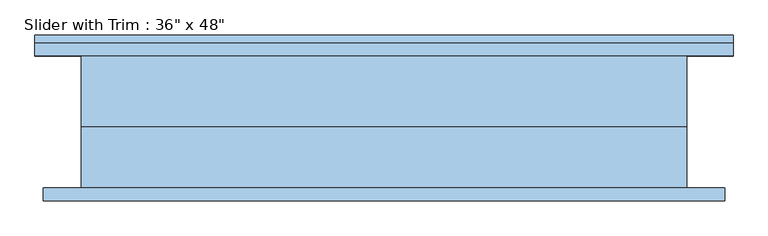
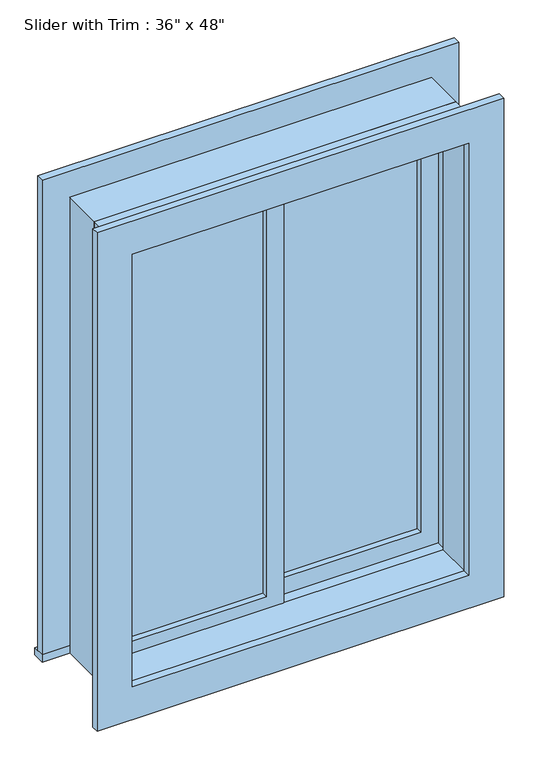
"""IFC4 building model written with IfcOpenShell, lengths in millimetres: window geometry."""

from ifc_helpers import new_model, si_unit, frame, origin, place, context, project, spatial, polyline, outline, extrude, source, transform, mapped, element, save


def window_242facca(model_context):
    return source(origin(), model_context, "Body", "SweptSolid", [
        extrude(outline(polyline([(-393.7, 20.625), (-22.225, 20.625), (-22.225, 7.925), (-393.7, 7.925), (-393.7, 20.625)])), frame((0.0, 0.0, 977.9), z_axis=(0.0, 0.0, 1.0), x_axis=(1.0, 0.0, 0.0)), (0.0, 0.0, 1.0), 1092.2),
        extrude(outline(polyline([(2114.55, -438.15), (933.45, -438.15), (933.45, 22.225), (2114.55, 22.225), (2114.55, -438.15)]), holes=[polyline([(2070.1, -393.7), (2070.1, -22.225), (977.9, -22.225), (977.9, -393.7), (2070.1, -393.7)])]), frame((0.0, -7.95, 0.0), z_axis=(0.0, 1.0, 0.0), x_axis=(0.0, 0.0, 1.0)), (0.0, 0.0, 1.0), 44.45),
        extrude(outline(polyline([(-527.05, 131.75), (527.05, 131.75), (527.05, 100.0), (-527.05, 100.0), (-527.05, 131.75)])), frame((0.0, 0.0, 914.4), z_axis=(0.0, 0.0, 1.0), x_axis=(1.0, 0.0, 0.0)), (0.0, 0.0, 1.0), 19.05),
        extrude(outline(polyline([(2114.55, -438.15), (2114.55, 438.15), (933.45, 438.15), (933.45, 527.05), (2203.45, 527.05), (2203.45, -527.05), (933.45, -527.05), (933.45, -438.15), (2114.55, -438.15)])), frame((0.0, 100.0, 0.0), z_axis=(0.0, 1.0, 0.0), x_axis=(0.0, 0.0, 1.0)), (0.0, 0.0, 1.0), 19.05),
        extrude(outline(polyline([(2190.75, 514.35), (2190.75, -514.35), (857.25, -514.35), (857.25, 514.35), (2190.75, 514.35)]), holes=[polyline([(2101.85, 425.45), (946.15, 425.45), (946.15, -425.45), (2101.85, -425.45), (2101.85, 425.45)])]), frame((0.0, -119.05, 0.0), z_axis=(0.0, 1.0, 0.0), x_axis=(0.0, 0.0, 1.0)), (0.0, 0.0, 1.0), 19.05),
        extrude(outline(polyline([(393.7, 52.375), (22.225, 52.375), (22.225, 65.075), (393.7, 65.075), (393.7, 52.375)])), frame((0.0, 0.0, 977.9), z_axis=(0.0, 0.0, 1.0), x_axis=(1.0, 0.0, 0.0)), (0.0, 0.0, 1.0), 1092.2),
        extrude(outline(polyline([(2114.55, -22.225), (933.45, -22.225), (933.45, 438.15), (2114.55, 438.15), (2114.55, -22.225)]), holes=[polyline([(2070.1, 22.225), (2070.1, 393.7), (977.9, 393.7), (977.9, 22.225), (2070.1, 22.225)])]), frame((0.0, 36.5, 0.0), z_axis=(0.0, 1.0, 0.0), x_axis=(0.0, 0.0, 1.0)), (0.0, 0.0, 1.0), 44.45),
        extrude(outline(polyline([(2133.6, -457.2), (914.4, -457.2), (914.4, 457.2), (2133.6, 457.2), (2133.6, -457.2)]), holes=[polyline([(2101.85, -425.45), (2101.85, 425.45), (946.15, 425.45), (946.15, -425.45), (2101.85, -425.45)])]), frame((0.0, -100.0, 0.0), z_axis=(0.0, 1.0, 0.0), x_axis=(0.0, 0.0, 1.0)), (0.0, 0.0, 1.0), 92.05),
        extrude(outline(polyline([(2133.6, 457.2), (2133.6, -457.2), (914.4, -457.2), (914.4, 457.2), (2133.6, 457.2)]), holes=[polyline([(2114.55, 438.15), (933.45, 438.15), (933.45, -438.15), (2114.55, -438.15), (2114.55, 438.15)])]), frame((0.0, -7.95, 0.0), z_axis=(0.0, 1.0, 0.0), x_axis=(0.0, 0.0, 1.0)), (0.0, 0.0, 1.0), 107.95),
    ])


if __name__ == "__main__":
    model = new_model("IFC4")
    model_context = context("Model", 3, world=origin())
    ifc_project = project(units=[si_unit("LENGTHUNIT", "METRE", prefix="MILLI")], contexts=[model_context])
    site = spatial("IfcSite", under=ifc_project)
    building = spatial("IfcBuilding", under=site)
    placement = place(None, origin())
    window_shape = window_242facca(model_context)
    element("IfcWindow", 1, ObjectType="Slider with Trim : 36\" x 48\"", at=placement, inside=building, context=model_context, shape_type="MappedRepresentation", body=[
        mapped(window_shape, transform((0.0, 0.0, 0.0), x_axis=(1.0, 0.0, 0.0), y_axis=(0.0, 1.0, 0.0), z_axis=(0.0, 0.0, 1.0))),
    ])
    save(model, "model.ifc")

# Revit data of these elements
# Type "Slider with Trim : 36\" x 48\""
#   Type Mark = "19"
#   Construction Type Id = "GSP4R"
#   Assembly Code = "B2020100"
#   Analytic Construction = "1/8 in Pilkington single glazing"
#   Visual Light Transmittance = 0.9
#   Solar Heat Gain Coefficient = 0.78
#   Heat Transfer Coefficient (U) = 3.6886 W/(m²·K)
#   Height = 1219.2 mm
#   Default Sill Height = 914.4 mm
#   Trim Projection - Ext. = 19.05 mm
#   Trim Projection - Int. = 19.05 mm
#   Trim Width - Exterior = 88.9 mm
#   Trim Width - Interior = 88.9 mm
#   Width = 914.4 mm
#   Window Inset = 19.05 mm
#   Define Thermal Properties by = 1
#   Glass Pane Material = Glass
#   Sash Material = Sash
#   Trim Exterior Material = Trim
#   Trim Interior Material = Trim
#   Wall Closure = (empty or 0)
# Element 1 (IfcWindow, "Slider with Trim : 36\" x 48\"")
#   Materials on its faces: "Sash", "Trim", "Glass"
# Materials
#   "Glass": class "Glass", colour RGB 218 227 224, transparency 0.85, Description = "Soda Lime Glass", Cost = 0
#   "Sash": class "Wood", colour RGB 136 99 55, transparency 0
#   "Trim": class "Wood", colour RGB 224 178 126, transparency 0
